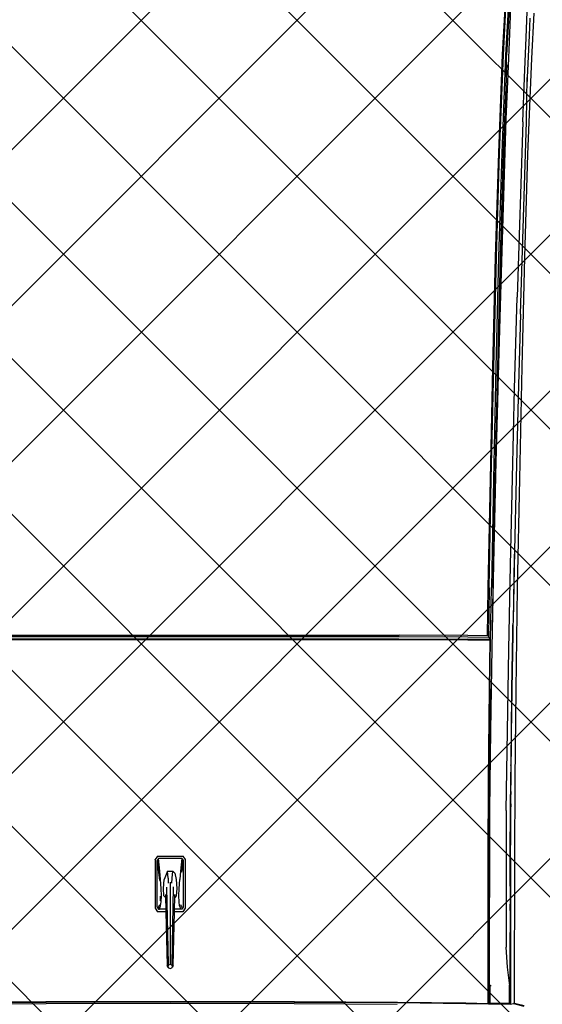
# Model space of a CAD drawing. Units: inches. Extents: x 2167 to 2589, y 1680 to 2489.
# Tile 8 of 38: x 2275 to 2299, y 1727 to 1771. Entities that reach past the tile are written whole.
import ezdxf

# ---------------------------------------------------------------- set-up
doc = ezdxf.new("R2010")
doc.units = ezdxf.units.IN
doc.header["$MEASUREMENT"] = 0
doc.layers.get('0').update_dxf_attribs({"color": 250})
doc.layers.add('C-PRKG-VEHS', color=8, linetype='Continuous', lineweight=13)
doc.layers.add('L-PVMT-PATT', color=252, linetype='Continuous', lineweight=13)
doc.layers.add('Edges', color=250, linetype='Continuous')

# ---------------------------------------------------------------- blocks, each defined once
blk = doc.blocks.new('Nissan Qashqai pl')
at = {"layer": 'Edges'}
for p, q in [((9.5168, 12.4903), (9.4761, 12.4919)), ((9.4782, 12.5024), (9.5503, 12.4987)), ((9.4862, 12.4961), (9.514, 12.4949)), ((9.514, 12.4949), (9.5811, 12.492)), ((9.5812, 12.4874), (9.5168, 12.4903)), ((9.5503, 12.4987), (9.7029, 12.4926)), ((9.651, 12.4906), (9.5811, 12.492)), ((9.5811, 12.492), (9.594, 12.4914)), ((9.6514, 12.4849), (9.5812, 12.4874)), ((9.9583, 12.4812), (9.651, 12.4906)), ((9.7029, 12.4926), (9.8673, 12.4878)), ((9.8673, 12.4878), (10.0423, 12.4835)), ((9.6514, 12.4849), (9.9312, 12.4761)), ((10.0776, 12.4719), (9.9312, 12.4761)), ((9.9583, 12.4812), (10.091, 12.4775)), ((10.0423, 12.4835), (10.2211, 12.4795)), ((10.2201, 12.4683), (10.0776, 12.4719)), ((10.091, 12.4775), (10.2202, 12.4743)), ((10.2202, 12.4743), (10.2203, 12.4743)), ((10.2203, 12.4743), (10.3353, 12.4717)), ((10.2211, 12.4795), (10.3955, 12.4762)), ((10.3353, 12.4717), (10.4477, 12.4694)), ((10.3353, 12.4717), (10.346, 12.4714)), ((10.3955, 12.4762), (10.5572, 12.4737)), ((10.5572, 12.4737), (10.7004, 12.4722)), ((10.7004, 12.4722), (10.8279, 12.4715)), ((11.0575, 12.4714), (11.0581, 12.4738)), ((11.0581, 12.4738), (11.0614, 12.4872)), ((11.0582, 12.47), (11.0624, 12.4866)), ((9.4694, 12.4654), (9.5105, 12.4637)), ((9.4706, 12.4561), (9.5443, 12.4522)), ((9.5446, 12.4542), (9.4709, 12.4581)), ((9.472, 12.463), (9.5454, 12.4591)), ((9.472, 12.4614), (9.5454, 12.4576)), ((9.5105, 12.4637), (9.5755, 12.4608)), ((9.5454, 12.4591), (9.5454, 12.4593)), ((9.5695, 12.4589), (9.5454, 12.4591)), ((9.5454, 12.4576), (9.7014, 12.4513)), ((9.5609, 12.4593), (9.5695, 12.4589)), ((9.5786, 12.4588), (9.5695, 12.4589)), ((9.5695, 12.4589), (9.7014, 12.4536)), ((9.5755, 12.4608), (9.6472, 12.4581)), ((9.6206, 12.4581), (9.5786, 12.4588)), ((9.6714, 12.4567), (9.6206, 12.4581)), ((9.6414, 12.458), (9.6407, 12.458)), ((9.6472, 12.4581), (9.9278, 12.4492)), ((9.6549, 12.4576), (9.6558, 12.4574)), ((9.6825, 12.4564), (9.6714, 12.4567)), ((9.6825, 12.4564), (9.6829, 12.4563)), ((9.6943, 12.456), (9.6825, 12.4564)), ((9.6943, 12.4558), (9.6943, 12.456)), ((9.6951, 12.456), (9.6943, 12.456)), ((9.6951, 12.4558), (9.6951, 12.456)), ((9.8565, 12.451), (9.6951, 12.456)), ((10.3586, 12.4651), (10.2201, 12.4683)), ((10.346, 12.4714), (10.4477, 12.4694)), ((10.4931, 12.4624), (10.3586, 12.4651)), ((10.4477, 12.4694), (10.4538, 12.4693)), ((10.4538, 12.4693), (10.4681, 12.469)), ((10.4676, 12.4691), (10.4538, 12.4693)), ((10.5566, 12.4677), (10.4676, 12.4691)), ((10.4676, 12.4691), (10.546, 12.4677)), ((10.4681, 12.469), (10.5866, 12.467)), ((10.6237, 12.4603), (10.4931, 12.4624)), ((10.546, 12.4677), (10.546, 12.4678)), ((10.546, 12.4677), (10.5576, 12.4675)), ((10.7, 12.4662), (10.5566, 12.4677)), ((10.5576, 12.4675), (10.6649, 12.4659)), ((10.5866, 12.467), (10.6649, 12.4659)), ((10.7502, 12.4586), (10.6237, 12.4603)), ((10.6649, 12.4659), (10.6786, 12.4658)), ((10.6649, 12.4659), (10.6772, 12.4657)), ((10.6786, 12.4657), (10.6772, 12.4657)), ((10.6786, 12.4658), (10.6786, 12.4662)), ((10.6786, 12.4657), (10.6786, 12.4658)), ((10.6786, 12.4658), (10.6801, 12.4657)), ((10.6786, 12.4657), (10.6801, 12.4657)), ((10.6801, 12.4662), (10.6801, 12.4657)), ((10.6801, 12.4657), (10.6801, 12.4657)), ((10.6801, 12.4657), (10.6811, 12.4657)), ((10.6801, 12.4657), (10.6811, 12.4657)), ((10.6811, 12.4662), (10.6811, 12.4657)), ((10.6811, 12.4657), (10.6811, 12.4657)), ((10.6811, 12.4657), (10.6966, 12.4654)), ((10.6811, 12.4657), (10.6991, 12.4655)), ((10.6811, 12.4657), (10.6991, 12.4655)), ((10.6966, 12.4654), (10.7144, 12.4653)), ((10.6991, 12.4655), (10.7144, 12.4653)), ((10.7201, 12.4661), (10.7, 12.4662)), ((10.7144, 12.4653), (10.7239, 12.4653)), ((10.7201, 12.4661), (10.7306, 12.4653)), ((10.7395, 12.4659), (10.7201, 12.4661)), ((10.7239, 12.4653), (10.7248, 12.4653)), ((10.7306, 12.4653), (10.7248, 12.4653)), ((10.7311, 12.4652), (10.7306, 12.4653)), ((10.7495, 12.4652), (10.7311, 12.4652)), ((10.7311, 12.4652), (10.7502, 12.4651)), ((10.7395, 12.4659), (10.7495, 12.4652)), ((10.7923, 12.4656), (10.7395, 12.4659)), ((10.8179, 12.4648), (10.7495, 12.4652)), ((10.7502, 12.4651), (10.7504, 12.4651)), ((10.7502, 12.4586), (10.968, 12.4585)), ((10.7504, 12.4651), (10.7808, 12.4649)), ((10.7808, 12.4649), (10.8179, 12.4648)), ((10.7923, 12.4652), (10.7923, 12.4656)), ((10.7933, 12.4656), (10.7923, 12.4656)), ((10.7933, 12.4652), (10.7933, 12.4656)), ((10.804, 12.4656), (10.7933, 12.4656)), ((10.804, 12.4653), (10.804, 12.4656)), ((10.8075, 12.4655), (10.804, 12.4656)), ((10.8075, 12.4655), (10.8075, 12.4653)), ((10.811, 12.4655), (10.8075, 12.4655)), ((10.811, 12.4655), (10.811, 12.4653)), ((10.8145, 12.4655), (10.811, 12.4655)), ((10.8145, 12.4653), (10.8145, 12.4655)), ((10.8279, 12.4654), (10.8145, 12.4655)), ((10.8277, 12.4647), (10.8179, 12.4648)), ((10.8711, 12.4646), (10.8277, 12.4647)), ((10.8279, 12.4715), (11.0544, 12.4714)), ((10.8279, 12.4654), (11.0592, 12.4653)), ((10.8711, 12.4646), (10.8824, 12.4646)), ((10.8824, 12.4646), (10.8825, 12.4646)), ((10.8825, 12.4646), (10.8884, 12.4646)), ((10.8884, 12.4646), (10.8923, 12.4646)), ((10.8923, 12.4646), (10.8996, 12.4646)), ((10.9097, 12.4646), (10.8996, 12.4646)), ((10.9097, 12.4646), (10.9399, 12.4646)), ((10.9399, 12.4646), (10.9491, 12.4645)), ((10.9491, 12.4645), (11.0301, 12.4645)), ((11, 12.4605), (10.968, 12.4585)), ((11.0301, 12.4645), (11, 12.4605)), ((11.0301, 12.4637), (11.0287, 12.4637)), ((11.03, 12.4635), (11.0301, 12.4637)), ((11.0301, 12.4642), (11.0301, 12.4645)), ((11.0574, 12.4637), (11.0301, 12.4637)), ((11.0544, 12.4714), (11.0575, 12.4714)), ((11.0568, 12.4323), (11.0574, 12.4637)), ((11.0574, 12.4637), (11.0592, 12.4653)), ((11.0575, 12.4714), (11.0582, 12.47)), ((11.0592, 12.4653), (11.0582, 12.47)), ((11.0585, 12.43), (11.0592, 12.4653)), ((9.5443, 12.4522), (9.701, 12.4459)), ((9.7011, 12.4478), (9.5446, 12.4542)), ((9.701, 12.4459), (9.8673, 12.441)), ((9.8673, 12.443), (9.7011, 12.4478)), ((9.7014, 12.4536), (9.8673, 12.4488)), ((9.7014, 12.4513), (9.8673, 12.4464)), ((9.9794, 12.4475), (9.8565, 12.451)), ((9.8673, 12.4488), (10.0429, 12.4444)), ((9.8673, 12.4464), (10.0429, 12.4421)), ((10.043, 12.4387), (9.8673, 12.443)), ((9.8673, 12.441), (10.0431, 12.4367)), ((9.9278, 12.4492), (10.0747, 12.445)), ((10.0998, 12.4443), (9.9794, 12.4475)), ((10.0429, 12.4444), (10.2216, 12.4404)), ((10.0429, 12.4421), (10.2215, 12.4381)), ((10.0747, 12.445), (10.078, 12.4449)), ((10.078, 12.4449), (10.2146, 12.4414)), ((10.2146, 12.4414), (10.0998, 12.4443)), ((10.2146, 12.4414), (10.2175, 12.4413)), ((10.2175, 12.4413), (10.3564, 12.4382)), ((10.2216, 12.4404), (10.3947, 12.4371)), ((10.2218, 12.4347), (10.043, 12.4387)), ((10.0431, 12.4367), (10.2218, 12.4327)), ((10.2215, 12.4381), (10.3945, 12.4348)), ((10.3947, 12.4314), (10.2218, 12.4347)), ((10.2218, 12.4327), (10.3947, 12.4294)), ((10.3564, 12.4382), (10.4638, 12.436)), ((10.4773, 12.4335), (10.3945, 12.4348)), ((10.3947, 12.4371), (10.4638, 12.436)), ((10.3947, 12.4314), (10.4735, 12.4301)), ((10.3947, 12.4294), (10.4715, 12.4282)), ((10.4638, 12.436), (10.4914, 12.4355)), ((10.4715, 12.4282), (10.4711, 12.3973)), ((10.4731, 12.3973), (10.4735, 12.4301)), ((10.4735, 12.4301), (10.4773, 12.4335)), ((10.4773, 12.4296), (10.4769, 12.3968)), ((10.4773, 12.4335), (10.4773, 12.4296)), ((10.4785, 12.433), (10.4773, 12.4335)), ((10.5561, 12.4323), (10.4773, 12.4335)), ((10.4781, 12.3972), (10.4785, 12.433)), ((10.5563, 12.4318), (10.4785, 12.433)), ((10.4914, 12.4355), (10.6223, 12.4333)), ((10.5561, 12.4323), (10.6996, 12.4308)), ((10.6999, 12.4304), (10.5563, 12.4318)), ((10.6223, 12.4333), (10.7493, 12.4316)), ((10.6996, 12.4308), (10.7722, 12.4304)), ((10.827, 12.4297), (10.6999, 12.4304)), ((10.7493, 12.4316), (11.0294, 12.4315)), ((10.7722, 12.4304), (10.7722, 12.4302)), ((10.7722, 12.4304), (10.7889, 12.4303)), ((10.7889, 12.4302), (10.7889, 12.4303)), ((10.7889, 12.4303), (10.7923, 12.4303)), ((10.7923, 12.4302), (10.7923, 12.4303)), ((10.7923, 12.4303), (10.7933, 12.4303)), ((10.7933, 12.4302), (10.7933, 12.4303)), ((10.7933, 12.4303), (10.8267, 12.4301)), ((10.8267, 12.4301), (11.0585, 12.43)), ((10.9133, 12.4296), (10.827, 12.4297)), ((10.9133, 12.4296), (10.9133, 12.4298)), ((10.9137, 12.4296), (10.9133, 12.4296)), ((10.9137, 12.4296), (10.9138, 12.4298)), ((10.9715, 12.4296), (10.9137, 12.4296)), ((10.9715, 12.4299), (10.9715, 12.4296)), ((11.0579, 12.4296), (10.9715, 12.4296)), ((11.0281, 12.4323), (11.0568, 12.4323)), ((11.0294, 12.4315), (11.0294, 12.4316)), ((11.0295, 12.4341), (11.0295, 12.4343)), ((11.0568, 12.4323), (11.0585, 12.43)), ((11.0572, 12.3942), (11.0579, 12.4296)), ((11.0579, 12.3938), (11.0585, 12.43)), ((11.0579, 12.4296), (11.0585, 12.43)), ((10.4711, 12.3973), (10.4706, 12.2875)), ((10.4726, 12.2875), (10.4731, 12.3973)), ((10.4764, 12.2872), (10.4769, 12.3968)), ((10.4776, 12.2874), (10.4781, 12.3972)), ((11.056, 12.2851), (11.0572, 12.3942)), ((11.0566, 12.2849), (11.0579, 12.3938)), ((10.4706, 11.5566), (10.4706, 12.2875)), ((10.4726, 11.5567), (10.4726, 12.2875)), ((10.4764, 11.5569), (10.4764, 12.2872)), ((10.4776, 11.5567), (10.4776, 12.2874)), ((11.0551, 12.1203), (11.056, 12.2851)), ((11.0557, 12.1202), (11.0566, 12.2849)), ((11.0595, 12.2842), (11.0586, 12.1198)), ((11.0547, 11.9221), (11.0551, 12.1203)), ((11.0554, 11.9221), (11.0557, 12.1202)), ((11.0586, 12.1198), (11.0583, 11.9221)), ((10.8228, 11.9421), (10.8224, 11.9421)), ((10.8228, 11.9421), (10.8283, 11.9461)), ((10.8228, 11.9021), (10.8228, 11.9421)), ((10.827, 11.9408), (10.8301, 11.9431)), ((10.827, 11.9408), (10.827, 11.9033)), ((10.827, 11.9408), (10.8467, 11.9386)), ((10.8279, 11.9461), (10.8283, 11.9461)), ((10.8283, 11.9461), (10.906, 11.9461)), ((10.8483, 11.9406), (10.8301, 11.9431)), ((10.8301, 11.9431), (10.9043, 11.9431)), ((10.8467, 11.9386), (10.8603, 11.9373)), ((10.9035, 11.9403), (10.9008, 11.9391)), ((10.9057, 11.9384), (10.9021, 11.9372)), ((10.905, 11.9414), (10.9035, 11.9403)), ((10.9043, 11.9431), (10.9074, 11.9408)), ((10.9043, 11.9431), (10.905, 11.9414)), ((10.9074, 11.9393), (10.9057, 11.9384)), ((10.906, 11.9461), (10.9116, 11.9421)), ((10.9074, 11.9408), (10.9074, 11.9393)), ((10.9074, 11.9393), (10.9074, 11.9291)), ((10.9116, 11.9421), (10.9116, 11.929)), ((10.8467, 11.9263), (10.8501, 11.9295)), ((10.8467, 11.9178), (10.8467, 11.9263)), ((10.8579, 11.9255), (10.8467, 11.9263)), ((10.8501, 11.9295), (10.8603, 11.9316)), ((10.8662, 11.925), (10.8579, 11.9255)), ((10.8746, 11.9363), (10.8603, 11.9373)), ((10.8603, 11.9316), (10.8746, 11.9327)), ((10.8647, 11.9221), (10.996, 11.9221)), ((10.9946, 11.9254), (10.872, 11.9276)), ((10.8861, 11.9361), (10.8746, 11.9363)), ((10.8746, 11.9327), (10.8861, 11.9319)), ((10.889, 11.9296), (10.884, 11.9298)), ((10.8959, 11.9365), (10.8861, 11.9361)), ((10.8861, 11.9319), (10.889, 11.9296)), ((10.9074, 11.9291), (10.889, 11.9296)), ((10.9021, 11.9372), (10.8959, 11.9365)), ((10.9116, 11.929), (10.9074, 11.9291)), ((10.9973, 11.9268), (10.9116, 11.929)), ((10.9969, 11.9247), (10.9946, 11.9254)), ((10.9969, 11.9247), (10.996, 11.9221)), ((10.996, 11.9221), (10.9969, 11.9195)), ((10.999, 11.9258), (10.9969, 11.9247)), ((10.9973, 11.9268), (11.0001, 11.9254)), ((10.999, 11.9258), (10.9973, 11.9268)), ((11.0012, 11.9247), (10.999, 11.9258)), ((11.0012, 11.9247), (11.0001, 11.9254)), ((11.002, 11.9221), (11.0012, 11.9247)), ((11.0012, 11.9195), (11.002, 11.9221)), ((11.0551, 11.7239), (11.0547, 11.9221)), ((11.0557, 11.724), (11.0554, 11.9221)), ((11.0583, 11.9221), (11.0586, 11.7244)), ((10.8579, 11.9187), (10.8467, 11.9178)), ((10.8467, 11.9178), (10.8603, 11.9126)), ((10.8603, 11.9068), (10.8467, 11.9056)), ((10.8579, 11.9187), (10.8662, 11.9191)), ((10.8746, 11.9115), (10.8603, 11.9126)), ((10.8746, 11.9078), (10.8603, 11.9068)), ((10.8723, 11.9165), (10.9946, 11.9187)), ((10.8861, 11.9122), (10.8746, 11.9115)), ((10.8861, 11.908), (10.8746, 11.9078)), ((10.884, 11.9144), (10.889, 11.9145)), ((10.889, 11.9145), (10.8861, 11.9122)), ((10.8959, 11.9077), (10.8861, 11.908)), ((10.8871, 11.9063), (10.8944, 11.906)), ((10.889, 11.9145), (10.9074, 11.915)), ((10.9021, 11.9069), (10.8959, 11.9077)), ((10.9057, 11.9058), (10.9021, 11.9069)), ((10.9074, 11.915), (10.9116, 11.9151)), ((10.9074, 11.915), (10.9074, 11.9049)), ((10.9116, 11.9151), (10.9973, 11.9173)), ((10.9116, 11.9151), (10.9116, 11.9021)), ((10.9946, 11.9187), (10.9969, 11.9195)), ((10.9969, 11.9195), (10.999, 11.9184)), ((11.0001, 11.9187), (10.9973, 11.9173)), ((10.9973, 11.9173), (10.999, 11.9184)), ((10.999, 11.9184), (10.9996, 11.9187)), ((10.9996, 11.9187), (11.0012, 11.9195)), ((11.0001, 11.9187), (10.9996, 11.9187)), ((11.0012, 11.9195), (11.0001, 11.9187)), ((10.8224, 11.9021), (10.8228, 11.9021)), ((10.8228, 11.9021), (10.8283, 11.8981)), ((10.8467, 11.9056), (10.827, 11.9033)), ((10.827, 11.9033), (10.8301, 11.9011)), ((10.8283, 11.8981), (10.8279, 11.8981)), ((10.8283, 11.8981), (10.906, 11.8981)), ((10.8301, 11.9011), (10.8483, 11.9036)), ((10.9043, 11.9011), (10.8301, 11.9011)), ((10.8483, 11.9036), (10.8619, 11.905)), ((10.9008, 11.905), (10.9035, 11.9039)), ((10.9035, 11.9039), (10.905, 11.9028)), ((10.9043, 11.9011), (10.9074, 11.9033)), ((10.905, 11.9028), (10.9043, 11.9011)), ((10.9074, 11.9049), (10.9057, 11.9058)), ((10.906, 11.8981), (10.9116, 11.9021)), ((10.9074, 11.9033), (10.9074, 11.9049)), ((10.9074, 11.9033), (10.9074, 11.9048)), ((11.056, 11.559), (11.0551, 11.7239)), ((11.0566, 11.5593), (11.0557, 11.724)), ((11.0586, 11.7244), (11.0595, 11.5599))]:
    blk.add_line(p, q, dxfattribs=at)
blk = doc.blocks.new('car')
blk.add_blockref('Nissan Qashqai pl', (-9.7433, -11.9151))
blk = doc.blocks.new('carr')
blk.add_blockref('car', (0.5124, -0.007))

msp = doc.modelspace()

# ---------------------------------------------------------------- hatches: boundary and pattern name
at = {"layer": 'L-PVMT-PATT'}
h = msp.add_hatch(dxfattribs=at)
h.set_pattern_fill('ANSI37', color=256, scale=40)
h.paths.add_polyline_path([(2417.548, 1783.695), (2417.548, 1846.042), (2239.361, 1846.042), (2239.361, 1687.695), (2369.843, 1687.695), (2369.843, 1696.695), (2375.607, 1696.695), (2416.107, 1696.695), (2417.548, 1696.695)])

# ---------------------------------------------------------------- block references
at = {"layer": 'C-PRKG-VEHS', "xscale": 28.42784210623918, "yscale": 28.42784210623918, "zscale": 28.42784210623918, "rotation": 270}
msp.add_blockref('carr', (2281.736, 1778.659), dxfattribs=at)

doc.saveas('drawing.dxf')
